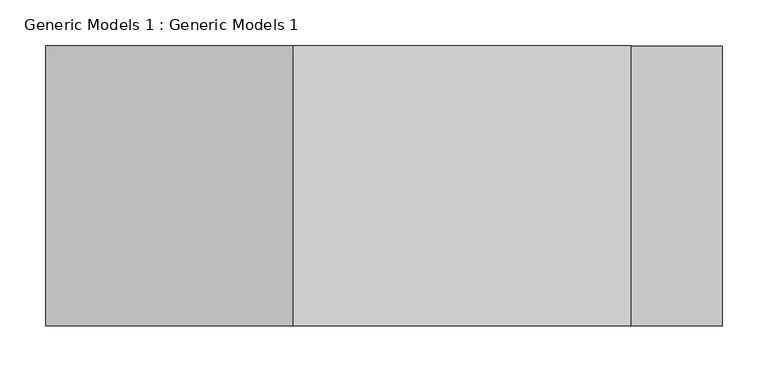
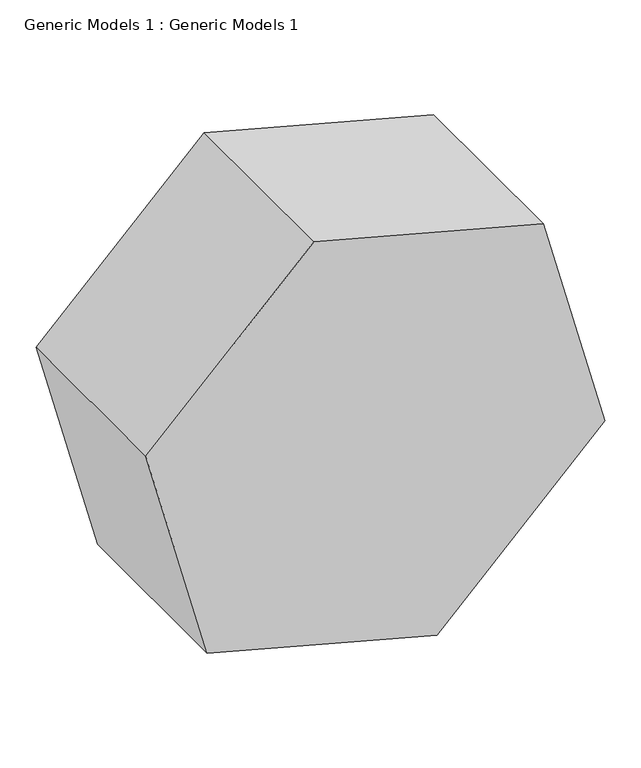
"""IFC4 building model written with IfcOpenShell, lengths in millimetres: proxy geometry, Generic Models 1 : Generic Models 1."""

from ifc_helpers import new_model, si_unit, frame, origin, place, context, project, spatial, polyline, outline, extrude, source, transform, mapped, element, save


def generic_models_1_generic_models_1_e32cbfde(model_context):
    return source(origin(), model_context, "Body", "SweptSolid", [
        extrude(outline(polyline([(904.7566299, -9949.4070438), (1003.366686, -10317.4247836), (733.9590024, -10586.8324672), (365.9412626, -10488.222411), (267.3312064, -10120.2046712), (536.73889, -9850.7969876), (904.7566299, -9949.4070438)])), frame((0.0, -9086.6225464, 0.0), z_axis=(0.0, 1.0, 0.0), x_axis=(0.0, 0.0, 1.0)), (0.0, 0.0, 1.0), 304.8),
    ])


if __name__ == "__main__":
    model = new_model("IFC4")
    model_context = context("Model", 3, world=origin())
    ifc_project = project(units=[si_unit("LENGTHUNIT", "METRE", prefix="MILLI")], contexts=[model_context])
    site = spatial("IfcSite", under=ifc_project)
    building = spatial("IfcBuilding", under=site)
    placement = place(None, origin())
    generic_models_1_generic_models_1_shape = generic_models_1_generic_models_1_e32cbfde(model_context)
    element("IfcBuildingElementProxy", 1, Name="Generic Models 1 : Generic Models 1", ObjectType="Generic Models 1 : Generic Models 1", at=placement, inside=building, context=model_context, shape_type="MappedRepresentation", body=[
        mapped(generic_models_1_generic_models_1_shape, transform((0.0, 0.0, 0.0), x_axis=(1.0, 0.0, 0.0), y_axis=(0.0, 1.0, 0.0), z_axis=(0.0, 0.0, 1.0))),
    ])
    save(model, "model.ifc")

# Revit data of these elements
# Element 1 (IfcBuildingElementProxy, "Generic Models 1 : Generic Models 1")
#   Materials on its faces: "Grass", "Carpet (1)"
# Materials
#   "Grass": class "Generic", colour RGB 104 137 66, transparency 0, Description = "Physical material.", Cost = 0
#   "Carpet (1)": class "Carpet", colour RGB 124 80 67, transparency 0, Description = "Interior finish", Cost = 0
